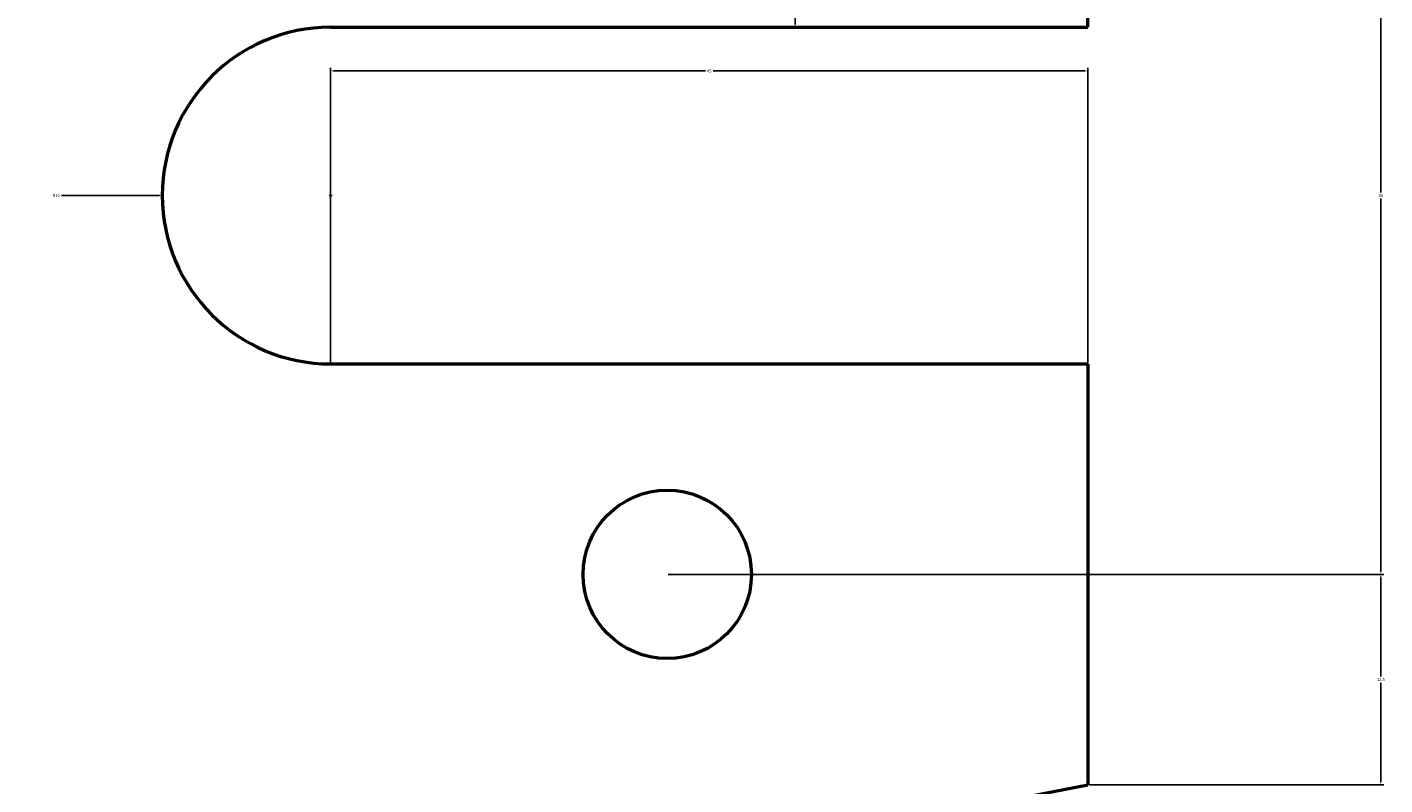
# Model space of a CAD drawing. Units: inches. Extents: x 457 to 775, y 319 to 541.
# Tile 10 of 12: x 694 to 775, y 376 to 421. Entities that reach past the tile are written whole.
import ezdxf

# ---------------------------------------------------------------- set-up
doc = ezdxf.new("R2010")
doc.units = ezdxf.units.IN
doc.header["$MEASUREMENT"] = 0
doc.layers.add('M-DIMS', color=2, linetype='Continuous', lineweight=18)
doc.layers.add('M-OUTL', color=7, linetype='Continuous', lineweight=50)
doc.styles.get("Standard").update_dxf_attribs({"font": 'arial.ttf'})
doc.dimstyles.get("Standard").update_dxf_attribs({"dimtxt": 0.18, "dimasz": 0.18, "dimexe": 0.18, "dimexo": 0.0625, "dimgap": 0.09, "dimtad": 0, "dimtih": 1, "dimtoh": 1, "dimdec": 4, "dimzin": 0, "dimdsep": 46, "dimtxsty": 'Standard', "dimcen": 0.09, "dimadec": 0, "dimazin": 0, "dimtfac": 1, "dimtdec": 4, "dimtofl": 0, "dimtmove": 0, "dimatfit": 3, "dimfxl": 1, "dimtolj": 1, "dimtzin": 0, "dimarcsym": 0})

# ---------------------------------------------------------------- blocks, each defined once
blk = doc.blocks.new('MOUNT-HOLE-D10')
blk.add_circle((5, 5), 5)
blk = doc.blocks.new('*D11')
at = {"layer": 'Defpoints', "color": 0, "transparency": 16777216}
for p in [(739.531, 445.696), (756.931, 445.696), (756.931, 420.696)]:
    blk.add_point(p, dxfattribs=at)
at = {"layer": 'M-DIMS', "color": 0, "lineweight": -2, "transparency": 16777216}
for p, q in [((756.869, 445.696), (739.351, 445.696)), ((739.531, 445.516), (739.531, 433.378)), ((739.531, 420.876), (739.531, 433.014)), ((756.869, 420.696), (739.351, 420.696))]:
    blk.add_line(p, q, dxfattribs=at)
at = {"layer": 'M-DIMS', "color": 0, "transparency": 16777216}
for points in [[(739.501, 445.516), (739.561, 445.516), (739.531, 445.696)], [(739.501, 420.876), (739.561, 420.876), (739.531, 420.696)]]:
    blk.add_solid(points, dxfattribs=at)
at = {"layer": 'M-DIMS', "color": 0, "transparency": 16777216, "insert": (739.531, 433.196), "char_height": 0.18, "attachment_point": 5}
blk.add_mtext('\\A1;25', dxfattribs=at)
blk = doc.blocks.new('*D12')
at = {"layer": 'Defpoints', "color": 0, "transparency": 16777216}
for p in [(756.931, 418.096), (711.931, 400.696), (756.931, 400.696)]:
    blk.add_point(p, dxfattribs=at)
at = {"layer": 'M-DIMS', "color": 0, "lineweight": -2, "transparency": 16777216}
for p, q in [((711.931, 400.759), (711.931, 418.276)), ((712.111, 418.096), (734.208, 418.096)), ((756.751, 418.096), (734.654, 418.096)), ((756.931, 400.759), (756.931, 418.276))]:
    blk.add_line(p, q, dxfattribs=at)
at = {"layer": 'M-DIMS', "color": 0, "transparency": 16777216}
for points in [[(712.111, 418.126), (712.111, 418.066), (711.931, 418.096)], [(756.751, 418.126), (756.751, 418.066), (756.931, 418.096)]]:
    blk.add_solid(points, dxfattribs=at)
at = {"layer": 'M-DIMS', "color": 0, "transparency": 16777216, "insert": (734.431, 418.096), "char_height": 0.18, "attachment_point": 5}
blk.add_mtext('\\A1;45', dxfattribs=at)
blk = doc.blocks.new('*D14')
at = {"layer": 'Defpoints', "color": 0, "transparency": 16777216}
for p in [(731.931, 433.196), (774.331, 433.196), (731.931, 388.196)]:
    blk.add_point(p, dxfattribs=at)
at = {"layer": 'M-DIMS', "color": 0, "lineweight": -2, "transparency": 16777216}
for p, q in [((731.994, 433.196), (774.511, 433.196)), ((774.331, 433.016), (774.331, 410.878)), ((774.331, 388.376), (774.331, 410.514)), ((731.994, 388.196), (774.511, 388.196))]:
    blk.add_line(p, q, dxfattribs=at)
at = {"layer": 'M-DIMS', "color": 0, "transparency": 16777216}
for points in [[(774.301, 433.016), (774.361, 433.016), (774.331, 433.196)], [(774.301, 388.376), (774.361, 388.376), (774.331, 388.196)]]:
    blk.add_solid(points, dxfattribs=at)
at = {"layer": 'M-DIMS', "color": 0, "transparency": 16777216, "insert": (774.331, 410.696), "char_height": 0.18, "attachment_point": 5}
blk.add_mtext('\\A1;45', dxfattribs=at)
blk = doc.blocks.new('*D15')
at = {"layer": 'Defpoints', "color": 0, "transparency": 16777216}
for p in [(731.931, 388.196), (756.931, 375.696), (774.331, 375.696)]:
    blk.add_point(p, dxfattribs=at)
at = {"layer": 'M-DIMS', "color": 0, "lineweight": -2, "transparency": 16777216}
for p, q in [((731.994, 388.196), (774.511, 388.196)), ((774.331, 388.016), (774.331, 382.128)), ((774.331, 375.876), (774.331, 381.764)), ((756.994, 375.696), (774.511, 375.696))]:
    blk.add_line(p, q, dxfattribs=at)
at = {"layer": 'M-DIMS', "color": 0, "transparency": 16777216}
for points in [[(774.301, 388.016), (774.361, 388.016), (774.331, 388.196)], [(774.301, 375.876), (774.361, 375.876), (774.331, 375.696)]]:
    blk.add_solid(points, dxfattribs=at)
at = {"layer": 'M-DIMS', "color": 0, "transparency": 16777216, "insert": (774.331, 381.946), "char_height": 0.18, "attachment_point": 5}
blk.add_mtext('\\A1;12.5', dxfattribs=at)
blk = doc.blocks.new('*D22')
at = {"layer": 'Defpoints', "color": 0, "transparency": 16777216}
for p in [(701.931, 410.696), (711.931, 410.696)]:
    blk.add_point(p, dxfattribs=at)
at = {"layer": 'M-DIMS', "color": 0, "lineweight": -2, "transparency": 16777216}
for p, q in [((695.931, 410.696), (701.751, 410.696)), ((711.841, 410.696), (712.021, 410.696)), ((711.931, 410.606), (711.931, 410.786))]:
    blk.add_line(p, q, dxfattribs=at)
at = {"layer": 'M-DIMS', "color": 0, "transparency": 16777216}
blk.add_solid([(701.751, 410.726), (701.751, 410.666), (701.931, 410.696)], dxfattribs=at)
at = {"layer": 'M-DIMS', "color": 0, "transparency": 16777216, "insert": (695.626, 410.696), "char_height": 0.18, "attachment_point": 5}
blk.add_mtext('\\A1;R10', dxfattribs=at)

msp = doc.modelspace()

# ---------------------------------------------------------------- linework, layer by layer
at = {"layer": 'M-OUTL'}
for p, q in [((756.931, 420.696), (756.931, 445.696)), ((711.931, 420.696), (756.931, 420.696)), ((711.931, 400.696), (756.931, 400.696)), ((756.931, 400.696), (756.931, 375.696)), ((554.931, 336.696), (756.931, 375.696))]:
    msp.add_line(p, q, dxfattribs=at)
msp.add_arc((711.931, 410.696), 10, 90, 270, dxfattribs=at)

# ---------------------------------------------------------------- block references
msp.add_blockref('MOUNT-HOLE-D10', (726.931, 383.196), dxfattribs=at)

# ---------------------------------------------------------------- dimensions: what is measured, and where the dimension line sits
at = {"layer": 'M-DIMS'}
for base, p1, p2, angle, override, picture, middle in [((739.531, 445.696), (756.931, 420.696), (756.931, 445.696), 90, {"dimdec": 0, "dimlfac": 1, "dimrnd": 0, "dimzin": 0, "dimdsep": 46, "dimlunit": 2}, '*D11', (739.531, 433.196)), ((774.331, 433.196), (731.931, 388.196), (731.931, 433.196), 90, {"dimdec": 0, "dimlfac": 1, "dimrnd": 0, "dimzin": 0, "dimdsep": 46, "dimlunit": 2}, '*D14', (774.331, 410.696)), ((756.931, 418.096), (711.931, 400.696), (756.931, 400.696), 0, {"dimdec": 0, "dimlfac": 1, "dimrnd": 0, "dimzin": 0, "dimdsep": 46, "dimlunit": 2}, '*D12', (734.431, 418.096)), ((774.331, 375.696), (731.931, 388.196), (756.931, 375.696), 90, {"dimdec": 1, "dimlfac": 1, "dimrnd": 0, "dimzin": 0, "dimdsep": 46, "dimlunit": 2}, '*D15', (774.331, 381.946))]:
    dim = msp.add_linear_dim(base=base, p1=p1, p2=p2, angle=angle, dimstyle='Standard', override=override, dxfattribs=at)
    dim.commit()
    dim.dimension.update_dxf_attribs({"geometry": picture, "text_midpoint": middle})
dim = msp.add_radius_dim(center=(711.931, 410.696), mpoint=(701.931, 410.696), dimstyle='Standard', override={"dimdec": 0, "dimlfac": 1, "dimrnd": 0, "dimzin": 0, "dimdsep": 46, "dimlunit": 2}, dxfattribs=at)
dim.commit()
dim.dimension.update_dxf_attribs({"geometry": '*D22', "text_midpoint": (695.931, 410.696), "dimtype": 164})

doc.saveas('drawing.dxf')
